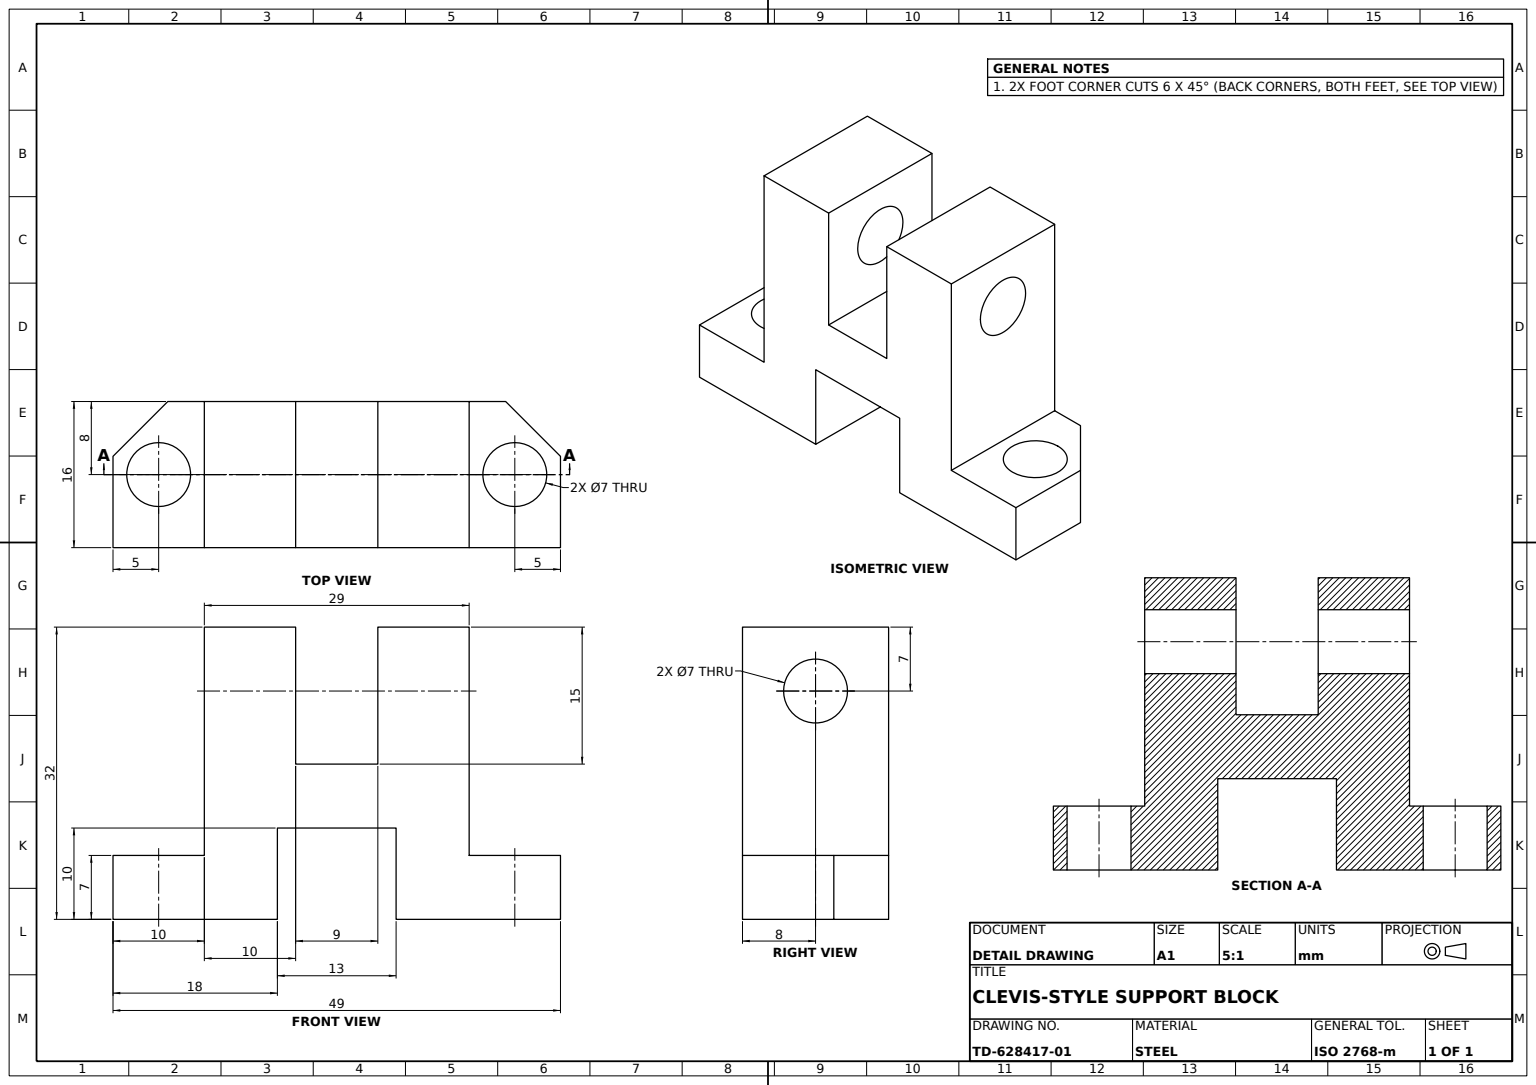
SolidWorks part; units mm, degrees
material "Plain Carbon Steel"
ref_plane "Front Plane" through (0, 0, 0) normal (0, 0, 1) x (1, 0, 0)
ref_plane "Top Plane" through (0, 0, 0) normal (0, 1, 0) x (1, 0, 0)
ref_plane "Right Plane" through (0, 0, 0) normal (1, 0, 0) x (0, 0, -1)
sketch "Base Profile Sketch" plane through (0, 0, 0) normal (0, 0, 1) x (1, 0, 0)
  line L1 (-14.5, -16) -> (14.5, -16)
  line L2 (-14.5, -16) -> (-14.5, 16)
  line L3 (-14.5, 16) -> (14.5, 16)
  line L4 (14.5, -16) -> (14.5, 16)
  line L5 (-14.5, -16) -> (14.5, 16) construction
  line L6 (-14.5, 16) -> (14.5, -16) construction
  point P0 (0, 0)
  dimension "D1" = 29
  dimension "D2" = 32
extrude "Base Block" add sketch "Base Profile Sketch" along normal blind 16
sketch "Centre Slot Sketch" plane through (0, 0, 16) normal (0, 0, 1) x (1, 0, 0)
  line L0 (0, 4.0137) -> (0, -26.691) construction
  line L1 (-6.5, -16) -> (6.5, -16)
  line L2 (-6.5, -16) -> (-6.5, -6)
  line L3 (-6.5, -6) -> (6.5, -6)
  line L4 (6.5, -16) -> (6.5, -6)
  line L5 (-6.5, -16) -> (6.5, -6) construction
  line L6 (-6.5, -6) -> (6.5, -16) construction
  line L8 (-14.5, -16) -> (14.5, -16) construction
  point P0 (0, -11)
  dimension "D1" = 13
  dimension "D2" = 10
extrude "Centre Slot" cut sketch "Centre Slot Sketch" against normal blind 16
sketch "Side Notch Sketch" plane through (0, 0, 16) normal (0, 0, 1) x (1, 0, 0)
  line L0 (14.5, 16) -> (-14.5, 16) construction
  line L1 (-4.5, 16) -> (4.5, 16)
  line L2 (-4.5, 16) -> (-4.5, 1)
  line L3 (-4.5, 1) -> (4.5, 1)
  line L4 (4.5, 16) -> (4.5, 1)
  line L5 (0, -11.1859) -> (0, 21.3491) construction
  dimension "D1" = 9
  dimension "D2" = 15
extrude "Side Notch" cut sketch "Side Notch Sketch" against normal through all
sketch "Foot Hole Sketch" plane through (14.5, 0, 0) normal (1, 0, 0) x (0, 0, -1)
  line L0 (-8, 16) -> (-8, 2.6062) construction
  line L1 (-16, 16) -> (0, 16) construction
  circle A0 centre (-8, 9) radius 3.5
  dimension "D1" = 7
  dimension "D2" = 7
extrude "Foot Hole" cut sketch "Foot Hole Sketch" against normal through all
sketch "Upright Lug 1 Sketch" plane through (0, -16, 0) normal (0, -1, 0) x (1, 0, 0)
  line L0 (-18.5, 0) -> (-24.5, 6)
  line L1 (-14.5, 0) -> (-18.5, 0)
  line L3 (-14.5, 16) -> (-24.5, 16)
  line L4 (-14.5, 0) -> (-6.5, 0)
  line L5 (-6.5, 0) -> (-6.5, 16)
  line L6 (-6.5, 16) -> (-14.5, 16)
  line L7 (-14.5, 16) -> (-14.5, 0)
  line L8 (-14.5, 0) -> (-6.5, 0)
  line L9 (-6.5, 0) -> (-6.5, 16)
  line L10 (-6.5, 16) -> (-14.5, 16)
  line L12 (-24.5, 6) -> (-24.5, 16)
  point P4 (-24.5, 0)
  dimension "D2" = 10
  dimension "D1" = 0
extrude "Upright Lug 1" add sketch "Upright Lug 1 Sketch" against normal blind 7
sketch "Upright Lug 2 Sketch" plane through (0, -16, 0) normal (0, -1, 0) x (1, 0, 0)
  line L0 (18.5, 0) -> (24.5, 6)
  line L1 (14.5, 0) -> (18.5, 0)
  line L3 (14.5, 16) -> (24.5, 16)
  line L4 (24.5, 6) -> (24.5, 16)
  line L8 (14.5, 16) -> (6.5, 16)
  line L9 (6.5, 16) -> (6.5, 0)
  line L10 (6.5, 0) -> (14.5, 0)
  line L11 (14.5, 0) -> (14.5, 16)
  line L12 (14.5, 16) -> (6.5, 16)
  line L13 (6.5, 16) -> (6.5, 0)
  line L14 (6.5, 0) -> (14.5, 0)
  point P3 (24.5, 0)
  dimension "D1" = 16
  dimension "D2" = 10
  dimension "D3" = 0
extrude "Upright Lug 2" add sketch "Upright Lug 2 Sketch" against normal blind 7 contours L0 L4 L3 L1
sketch "Lug 1 Cross Hole Sketch" plane through (0, -9, 0) normal (0, 1, 0) x (1, 0, 0)
  line L0 (-14.5, -8) -> (-24.5, -8) construction
  line L1 (-14.5, -16) -> (-14.5, 0) construction
  line L2 (-24.5, -16) -> (-24.5, -6) construction
  line L3 (-19.5, -16) -> (-19.5, 0) construction
  line L4 (-14.5, -16) -> (-24.5, -16) construction
  circle A0 centre (-19.5, -8) radius 3.5
  dimension "D1" = 7
extrude "Lug 1 Cross Hole" cut sketch "Lug 1 Cross Hole Sketch" against normal blind 7
sketch "Lug 2 Cross Hole Sketch" plane through (0, -9, 0) normal (0, 1, 0) x (1, 0, 0)
  line L0 (-19.5, -8) -> (24.5, -8) construction
  line L1 (24.5, -6) -> (24.5, -16) construction
  line L2 (19.5, -16) -> (19.5, 0) construction
  line L3 (14.5, -16) -> (24.5, -16) construction
  circle A0 centre (19.5, -8) radius 3.5
  dimension "D1" = 7
  dimension "D2" = 8
extrude "Lug 2 Cross Hole" cut sketch "Lug 2 Cross Hole Sketch" against normal blind 7
